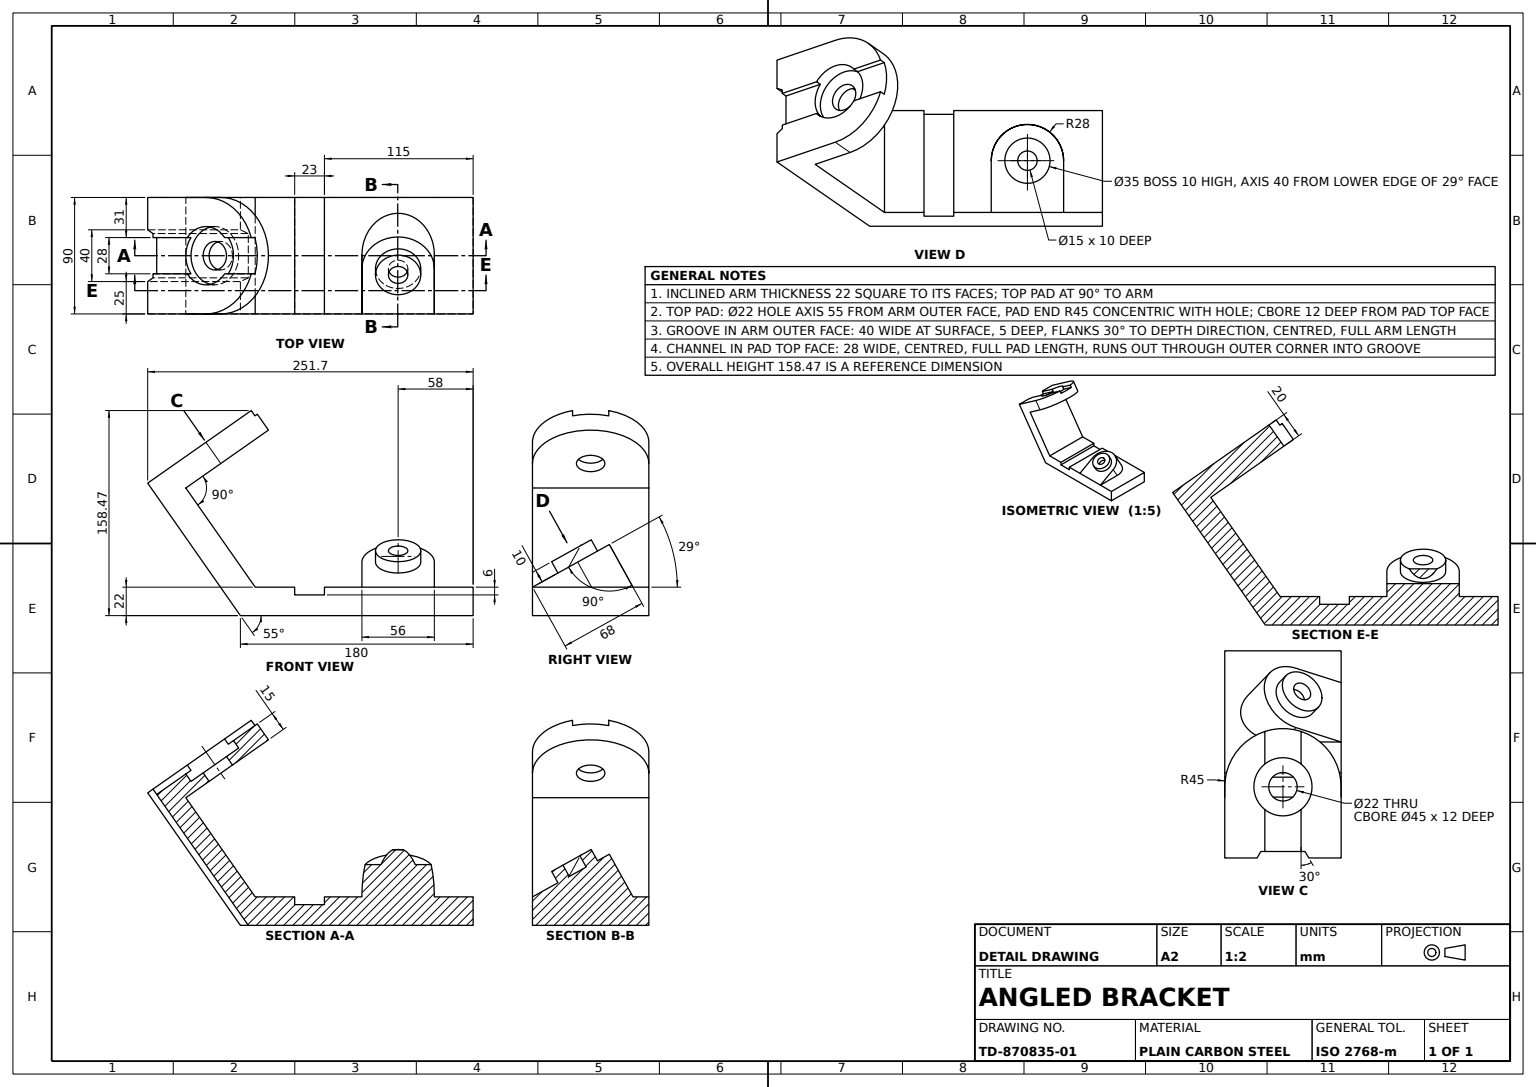
SolidWorks part; units mm, degrees
material "Plain Carbon Steel"
ref_plane "Front Plane" through (0, 0, 0) normal (0, 0, 1) x (1, 0, 0)
ref_plane "Top Plane" through (0, 0, 0) normal (0, 1, 0) x (1, 0, 0)
ref_plane "Right Plane" through (0, 0, 0) normal (1, 0, 0) x (0, 0, -1)
sketch "Base Plate Sketch" plane through (0, 0, 0) normal (0, 1, 0) x (1, 0, 0)
  line L1 (-90, -45) -> (90, -45)
  line L2 (-90, -45) -> (-90, 45)
  line L3 (-90, 45) -> (90, 45)
  line L4 (90, -45) -> (90, 45)
  line L5 (-90, -45) -> (90, 45) construction
  line L6 (-90, 45) -> (90, -45) construction
  point P0 (0, 0)
  dimension "D1" = 180
  dimension "D2" = 90
extrude "Base Plate 180x90x22" add sketch "Base Plate Sketch" along normal blind 22
ref_plane "Boss Axis Offset Plane" through (32, 0, 0) normal (1, 0, 0) x (0, 0, -1)
sketch "Inclined Boss Axis Sketch" plane through (32, 0, 0) normal (1, 0, 0) x (0, 0, -1)
  line L0 (-45, 22) -> (-10.0152, 41.3924) construction
  dimension "D1" = 40
  dimension "D2" = 29
ref_plane "Inclined Boss Plane" through (0, 35.9102, 19.9053) normal (0, -0.8746, -0.4848) x (-1, 0, 0)
sketch "Inclined Boss Block Sketch" plane through (0, 35.9102, 19.9053) normal (0, -0.8746, -0.4848) x (-1, 0, 0)
  line L0 (-32, -28.6921) -> (-32, 11.3079) construction
  line L1 (90, -28.6921) -> (-90, -28.6921) construction
  line L2 (-4, 11.3079) -> (-4, -28.6921)
  line L3 (-4, -28.6921) -> (-60, -28.6921)
  line L4 (-60, -28.6921) -> (-60, 11.3079)
  arc A0 (-4, 11.3079) -> (-60, 11.3079) centre (-32, 11.3079) ccw
  dimension "D1" = 56
  dimension "D2" = 40
extrude "Inclined Boss Block" add sketch "Inclined Boss Block Sketch" along normal up to next
sketch "Pivot Boss Sketch" plane through (0, 35.9102, 19.9053) normal (0, 0.8746, 0.4848) x (1, 0, 0)
  line L0 (32, -28.6921) -> (32, 11.3079) construction
  line L1 (60, -28.6921) -> (4, -28.6921) construction
  circle A0 centre (32, 11.3079) radius 17.5
  circle A1 centre (32, 11.3079) radius 7.5
  dimension "D1" = 35
  dimension "D3" = 15
  dimension "D2" = 40
extrude "Pivot Boss" add sketch "Pivot Boss Sketch" along normal blind 10
sketch "Cross Slot Sketch" plane through (0, 22, 0) normal (0, 1, 0) x (1, 0, 0)
  line L0 (90, 45) -> (-90, 45) construction
  line L1 (-48, 45) -> (-25, 45)
  line L2 (-48, 45) -> (-48, -45)
  line L3 (-48, -45) -> (-25, -45)
  line L4 (-25, 45) -> (-25, -45)
  line L5 (-90, -45) -> (4, -45) construction
  dimension "D1" = 23
  dimension "D2" = 85
extrude "Cross Slot 23x6" cut sketch "Cross Slot Sketch" against normal blind 6
sketch "Upright Arm Axis Sketch" plane through (0, 0, 45) normal (0, 0, 1) x (1, 0, 0)
  line L0 (-90, 0) -> (-161.6971, 102.394) construction
  dimension "D1" = 125
  dimension "D2" = 55
ref_plane "Upright Arm Plane" through (-60.3909, -42.2862, 0) normal (0.8192, 0.5736, 0) x (0, 0, -1)
sketch "Upright Arm Sketch" plane through (-60.3909, -42.2862, 0) normal (0.8192, 0.5736, 0) x (0, 0, -1)
  line L0 (-45, 51.6219) -> (-45, 176.6219) construction
  line L1 (-45, 51.6219) -> (45, 51.6219)
  line L2 (-45, 51.6219) -> (-45, 176.6219)
  line L3 (-45, 176.6219) -> (45, 176.6219)
  line L4 (45, 51.6219) -> (45, 176.6219)
  dimension "D1" = 90
  dimension "D2" = 125
  dimension "D3" = 51.6219
extrude "Inclined Upright Arm" add sketch "Upright Arm Sketch" along normal blind 22
sketch "Top Pad Sketch" plane through (-101.3061, 144.6802, 0) normal (-0.5736, 0.8192, 0) x (0.8192, 0.5736, 0)
  line L0 (-73.7237, 45) -> (-73.7237, -45) construction
  line L1 (-18.7237, 45) -> (-73.7237, 45)
  line L2 (-73.7237, 45) -> (-73.7237, -45)
  line L3 (-73.7237, -45) -> (-18.7237, -45)
  arc A0 (-18.7237, -45) -> (-18.7237, 45) centre (-18.7237, 0) ccw
  dimension "D1" = 90
  dimension "D2" = 55
  dimension "D3" = 0
extrude "Top Pad" add sketch "Top Pad Sketch" against normal blind 20
hole_wizard "C-Bore Hole Ø22" positions "Sketch11" profile "Sketch12" legacy
sketch "Sketch11" plane through (-101.3061, 144.6802, 0) normal (-0.5736, 0.8192, 0) x (0.8192, 0.5736, 0)
  point P0 (-18.7237, 0)
sketch "Sketch12" plane through (-116.6437, 133.9407, 0) normal (0, 0, 1) x (-0.8192, -0.5736, 0)
  line L0 (0, 0) -> (0, 22.198)
  line L1 (0, 22.198) -> (11, 22.198)
  line L2 (11, 22.198) -> (11, 12)
  line L3 (11, 12) -> (22.5, 12)
  line L4 (22.5, 12) -> (22.5, 0)
  line L5 (22.5, 0) -> (0, 0)
  line L6 (0, 110) -> (0, -10) construction
  dimension "Diameter" = 22
  dimension "Depth" = 25
  dimension "C-Bore Diameter" = 45
  dimension "C-Bore Depth" = 12
sketch "Top Pad Notch Sketch" plane through (-101.3061, 144.6802, 0) normal (-0.5736, 0.8192, 0) x (0.8192, 0.5736, 0)
  line L0 (-73.7237, 20) -> (-68.7237, 17.1132)
  line L1 (-73.7237, 45) -> (-73.7237, -45) construction
  line L2 (-73.7237, -20) -> (-68.7237, -17.1132)
  line L3 (-73.7237, 20) -> (-73.7237, -20)
  line L4 (-68.7237, 17.1132) -> (-68.7237, -17.1132)
  dimension "D1" = 25
  dimension "D2" = 5
  dimension "D3" = 30
  dimension "D4" = 25
  dimension "D5" = 5
  dimension "D6" = 30
extrude "Top Pad Notches" cut sketch "Top Pad Notch Sketch" against normal through all
sketch "Cross Recess Sketch" plane through (-101.3061, 144.6802, 0) normal (-0.5736, 0.8192, 0) x (0.8192, 0.5736, 0)
  line L0 (-68.7237, -17.1132) -> (-68.7237, 17.1132) construction
  line L1 (-68.7237, 14) -> (-36.3376, 14)
  line L2 (-68.7237, 14) -> (-68.7237, -14)
  line L3 (-68.7237, -14) -> (-36.3376, -14)
  line L4 (-36.3376, 14) -> (-36.3376, -14)
  line L6 (-1.1098, 14) -> (28.8902, 14)
  line L7 (-1.1098, 14) -> (-1.1098, -14)
  line L8 (-1.1098, -14) -> (28.8902, -14)
  line L9 (28.8902, 14) -> (28.8902, -14)
  circle A0 centre (-18.7237, 0) radius 22.5 construction
  dimension "D1" = 28
  dimension "D2" = 14
  dimension "D3" = 28
  dimension "D4" = 14
  dimension "D5" = 30
extrude "Cross Recess 5 Deep" cut sketch "Cross Recess Sketch" against normal blind 5
